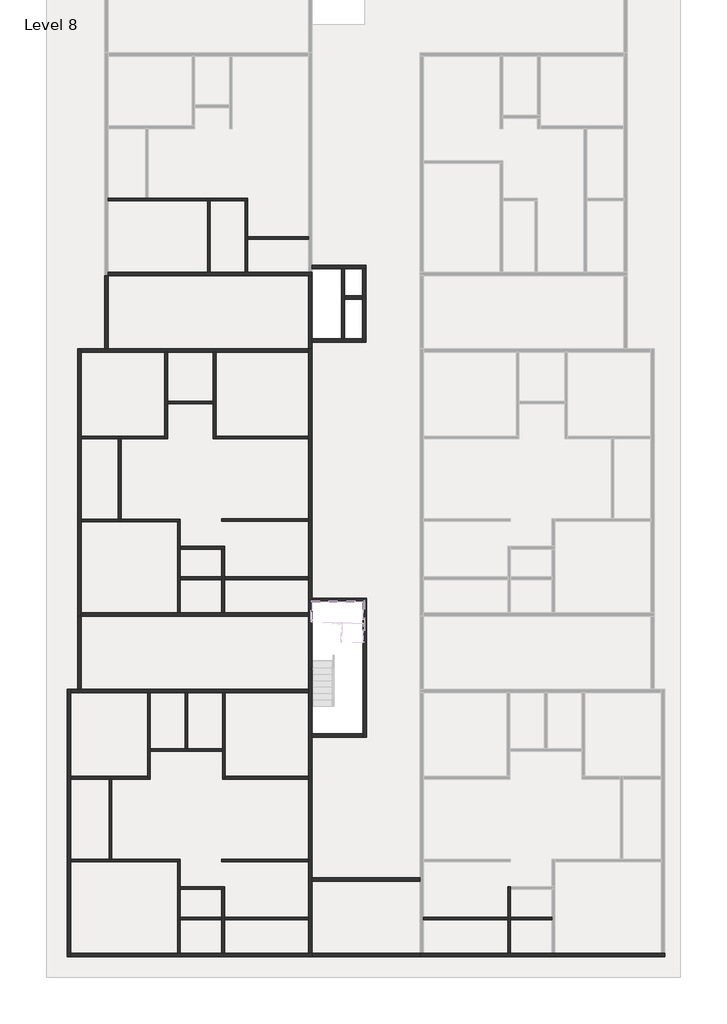
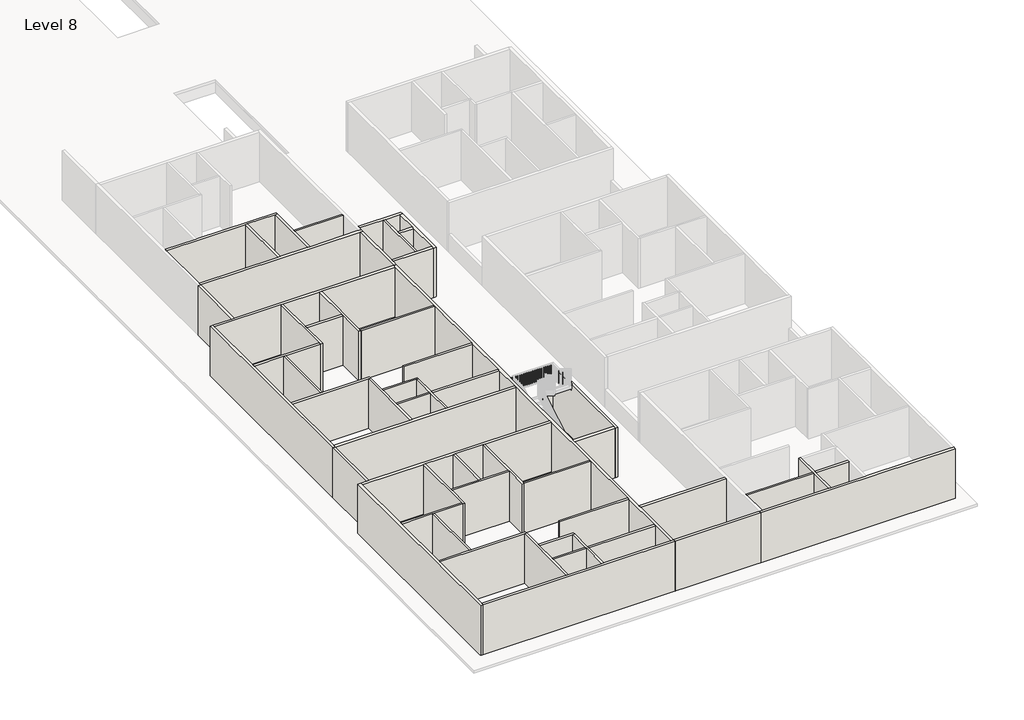
# One storey, part 1 of 8: 55 walls.
"""IFC4 building model written with IfcOpenShell, lengths in millimetres."""

from ifc_helpers import new_model, si_unit, frame, origin, place, context, project, spatial, polyline, outline, extrude, faceted_brep, element, save

model = new_model("IFC4")

# Units and contexts
model_context = context("Model", 3, world=origin())
ifc_project = project(units=[si_unit("LENGTHUNIT", "METRE", prefix="MILLI")], contexts=[model_context])

# Site, building, storey
site = spatial("IfcSite", under=ifc_project)
building = spatial("IfcBuilding", under=site)
storey = spatial("IfcBuildingStorey", under=building, Name="Level 8", Elevation=46570.6172466)

# Walls
placement = place(None, origin())
element("IfcWall", 1, ObjectType="4.5\"", at=placement, inside=storey, context=model_context, shape_type="Brep", body=[
    faceted_brep([(-12531.5544854, -1061.7344126, 46570.6172466), (-8188.1544854, -1061.7344126, 46570.6172466), (-8073.8544854, -1061.7344126, 46570.6172466), (-6549.8544854, -1061.7344126, 46570.6172466), (-6435.5544854, -1061.7344126, 46570.6172466), (-6435.5544854, -1061.7344126, 49618.6172466), (-6549.8544854, -1061.7344126, 49618.6172466), (-8073.8544854, -1061.7344126, 49618.6172466), (-8188.1544854, -1061.7344126, 49618.6172466), (-12531.5544854, -1061.7344126, 49618.6172466), (-12531.5544854, -947.4344126, 46570.6172466), (-12531.5544854, -947.4344126, 49618.6172466), (-10907.2415084, -947.4344126, 49618.6172466), (-10792.9415084, -947.4344126, 49618.6172466), (-6435.5544854, -947.4344126, 49618.6172466), (-6435.5544854, -947.4344126, 46570.6172466), (-10792.9415084, -947.4344126, 46570.6172466), (-10907.2415084, -947.4344126, 46570.6172466)], [[[0, 1, 2, 3, 4, 5, 6, 7, 8, 9]], [[10, 11, 12, 13, 14, 15, 16, 17]], [[4, 3, 2, 1, 0, 10, 17, 16, 15]], [[0, 9, 11, 10]], [[5, 4, 15, 14]], [[9, 8, 7, 6, 5, 14, 13, 12, 11]]]),
])
element("IfcWall", 2, ObjectType="4.5\"", at=placement, inside=storey, context=model_context, shape_type="Brep", body=[
    faceted_brep([(-6549.8544854, -1061.7344126, 46570.6172466), (-6549.8544854, -4185.9344126, 46570.6172466), (-6549.8544854, -4185.9344126, 49618.6172466), (-6549.8544854, -1061.7344126, 49618.6172466), (-6435.5544854, -1061.7344126, 46570.6172466), (-6435.5544854, -1061.7344126, 49618.6172466), (-6435.5544854, -2623.8344126, 49618.6172466), (-6435.5544854, -2738.1344126, 49618.6172466), (-6435.5544854, -4185.9344126, 49618.6172466), (-6435.5544854, -4185.9344126, 46570.6172466), (-6435.5544854, -2738.1344126, 46570.6172466), (-6435.5544854, -2623.8344126, 46570.6172466)], [[[0, 1, 2, 3]], [[4, 5, 6, 7, 8, 9, 10, 11]], [[1, 0, 4, 11, 10, 9]], [[0, 3, 5, 4]], [[2, 1, 9, 8]], [[3, 2, 8, 7, 6, 5]]]),
])
element("IfcWall", 3, ObjectType="4.5\"", at=placement, inside=storey, context=model_context, shape_type="SweptSolid", body=[
    extrude(outline(polyline([(-8188.1544854, -4185.9344126), (-8188.1544854, -1061.7344126), (-8073.8544854, -1061.7344126), (-8073.8544854, -4185.9344126), (-8188.1544854, -4185.9344126)])), frame((0.0, 0.0, 46570.6172466), z_axis=(0.0, 0.0, 1.0), x_axis=(1.0, 0.0, 0.0)), (0.0, 0.0, 1.0), 3048.0),
])
element("IfcWall", 4, ObjectType="4.5\"", at=placement, inside=storey, context=model_context, shape_type="SweptSolid", body=[
    extrude(outline(polyline([(-6435.5544854, -2623.8344126), (-3769.8415084, -2623.8344126), (-3769.8415084, -2738.1344126), (-6435.5544854, -2738.1344126), (-6435.5544854, -2623.8344126)])), frame((0.0, 0.0, 46570.6172466), z_axis=(0.0, 0.0, 1.0), x_axis=(1.0, 0.0, 0.0)), (0.0, 0.0, 1.0), 3048.0),
])
element("IfcWall", 5, ObjectType="4.5\"", at=placement, inside=storey, context=model_context, shape_type="Brep", body=[
    faceted_brep([(-10061.4044854, -7691.1344126, 46570.6172466), (-10061.4044854, -11348.7344126, 46570.6172466), (-10061.4044854, -11463.0344126, 46570.6172466), (-10061.4044854, -11463.0344126, 49618.6172466), (-10061.4044854, -11348.7344126, 49618.6172466), (-10061.4044854, -7691.1344126, 49618.6172466), (-9947.1044854, -7691.1344126, 46570.6172466), (-9947.1044854, -7691.1344126, 49618.6172466), (-9947.1044854, -9824.7344126, 49618.6172466), (-9947.1044854, -9939.0344126, 49618.6172466), (-9947.1044854, -11463.0344126, 49618.6172466), (-9947.1044854, -11463.0344126, 46570.6172466), (-9947.1044854, -9939.0344126, 46570.6172466), (-9947.1044854, -9824.7344126, 46570.6172466)], [[[0, 1, 2, 3, 4, 5]], [[6, 7, 8, 9, 10, 11, 12, 13]], [[2, 1, 0, 6, 13, 12, 11]], [[0, 5, 7, 6]], [[3, 2, 11, 10]], [[5, 4, 3, 10, 9, 8, 7]]]),
])
element("IfcWall", 6, ObjectType="4.5\"", at=placement, inside=storey, context=model_context, shape_type="Brep", body=[
    faceted_brep([(-10061.4044854, -11348.7344126, 46570.6172466), (-13719.0044854, -11348.7344126, 46570.6172466), (-13719.0044854, -11348.7344126, 49618.6172466), (-10061.4044854, -11348.7344126, 49618.6172466), (-10061.4044854, -11463.0344126, 46570.6172466), (-10061.4044854, -11463.0344126, 49618.6172466), (-11980.3915084, -11463.0344126, 49618.6172466), (-12094.6915084, -11463.0344126, 49618.6172466), (-13719.0044854, -11463.0344126, 49618.6172466), (-13719.0044854, -11463.0344126, 46570.6172466), (-12094.6915084, -11463.0344126, 46570.6172466), (-11980.3915084, -11463.0344126, 46570.6172466)], [[[0, 1, 2, 3]], [[4, 5, 6, 7, 8, 9, 10, 11]], [[1, 0, 4, 11, 10, 9]], [[0, 3, 5, 4]], [[2, 1, 9, 8]], [[3, 2, 8, 7, 6, 5]]]),
])
element("IfcWall", 7, ObjectType="4.5\"", at=placement, inside=storey, context=model_context, shape_type="SweptSolid", body=[
    extrude(outline(polyline([(-12094.6915084, -14968.2344126), (-12094.6915084, -11463.0344126), (-11980.3915084, -11463.0344126), (-11980.3915084, -14968.2344126), (-12094.6915084, -14968.2344126)])), frame((0.0, 0.0, 46570.6172466), z_axis=(0.0, 0.0, 1.0), x_axis=(1.0, 0.0, 0.0)), (0.0, 0.0, 1.0), 3048.0),
])
element("IfcWall", 8, ObjectType="4.5\"", at=placement, inside=storey, context=model_context, shape_type="Brep", body=[
    faceted_brep([(-13719.0044854, -15095.2344126, 46570.6172466), (-9510.2415084, -15095.2344126, 46570.6172466), (-9395.9415084, -15095.2344126, 46570.6172466), (-9395.9415084, -15095.2344126, 49618.6172466), (-9510.2415084, -15095.2344126, 49618.6172466), (-13719.0044854, -15095.2344126, 49618.6172466), (-13719.0044854, -14980.9344126, 46570.6172466), (-13719.0044854, -14980.9344126, 49618.6172466), (-9395.9415084, -14980.9344126, 49618.6172466), (-9395.9415084, -14980.9344126, 46570.6172466)], [[[0, 1, 2, 3, 4, 5]], [[6, 7, 8, 9]], [[2, 1, 0, 6, 9]], [[0, 5, 7, 6]], [[3, 2, 9, 8]], [[5, 4, 3, 8, 7]]]),
])
element("IfcWall", 9, ObjectType="4.5\"", at=placement, inside=storey, context=model_context, shape_type="Brep", body=[
    faceted_brep([(-9510.2415084, -15095.2344126, 46570.6172466), (-9510.2415084, -19070.3344126, 46570.6172466), (-9510.2415084, -19070.3344126, 49618.6172466), (-9510.2415084, -15095.2344126, 49618.6172466), (-9395.9415084, -15095.2344126, 46570.6172466), (-9395.9415084, -15095.2344126, 49618.6172466), (-9395.9415084, -16174.7344126, 49618.6172466), (-9395.9415084, -16289.0344126, 49618.6172466), (-9395.9415084, -17508.2344126, 49618.6172466), (-9395.9415084, -17622.5344126, 49618.6172466), (-9395.9415084, -19070.3344126, 49618.6172466), (-9395.9415084, -19070.3344126, 46570.6172466), (-9395.9415084, -17622.5344126, 46570.6172466), (-9395.9415084, -17508.2344126, 46570.6172466), (-9395.9415084, -16289.0344126, 46570.6172466), (-9395.9415084, -16174.7344126, 46570.6172466)], [[[0, 1, 2, 3]], [[4, 5, 6, 7, 8, 9, 10, 11, 12, 13, 14, 15]], [[1, 0, 4, 15, 14, 13, 12, 11]], [[0, 3, 5, 4]], [[2, 1, 11, 10]], [[3, 2, 10, 9, 8, 7, 6, 5]]]),
])
element("IfcWall", 10, ObjectType="4.5\"", at=placement, inside=storey, context=model_context, shape_type="Brep", body=[
    faceted_brep([(-9395.9415084, -16289.0344126, 46570.6172466), (-7567.1415084, -16289.0344126, 46570.6172466), (-7452.8415084, -16289.0344126, 46570.6172466), (-7452.8415084, -16289.0344126, 49618.6172466), (-7567.1415084, -16289.0344126, 49618.6172466), (-9395.9415084, -16289.0344126, 49618.6172466), (-9395.9415084, -16174.7344126, 46570.6172466), (-9395.9415084, -16174.7344126, 49618.6172466), (-7452.8415084, -16174.7344126, 49618.6172466), (-7452.8415084, -16174.7344126, 46570.6172466)], [[[0, 1, 2, 3, 4, 5]], [[6, 7, 8, 9]], [[2, 1, 0, 6, 9]], [[0, 5, 7, 6]], [[3, 2, 9, 8]], [[5, 4, 3, 8, 7]]]),
])
element("IfcWall", 11, ObjectType="4.5\"", at=placement, inside=storey, context=model_context, shape_type="Brep", body=[
    faceted_brep([(-7567.1415084, -16289.0344126, 46570.6172466), (-7567.1415084, -17508.2344126, 46570.6172466), (-7567.1415084, -17622.5344126, 46570.6172466), (-7567.1415084, -19070.3344126, 46570.6172466), (-7567.1415084, -19070.3344126, 49618.6172466), (-7567.1415084, -17622.5344126, 49618.6172466), (-7567.1415084, -17508.2344126, 49618.6172466), (-7567.1415084, -16289.0344126, 49618.6172466), (-7452.8415084, -16289.0344126, 46570.6172466), (-7452.8415084, -16289.0344126, 49618.6172466), (-7452.8415084, -17508.2344126, 49618.6172466), (-7452.8415084, -17622.5344126, 49618.6172466), (-7452.8415084, -19070.3344126, 49618.6172466), (-7452.8415084, -19070.3344126, 46570.6172466), (-7452.8415084, -17622.5344126, 46570.6172466), (-7452.8415084, -17508.2344126, 46570.6172466)], [[[0, 1, 2, 3, 4, 5, 6, 7]], [[8, 9, 10, 11, 12, 13, 14, 15]], [[3, 2, 1, 0, 8, 15, 14, 13]], [[0, 7, 9, 8]], [[4, 3, 13, 12]], [[7, 6, 5, 4, 12, 11, 10, 9]]]),
])
element("IfcWall", 12, ObjectType="4.5\"", at=placement, inside=storey, context=model_context, shape_type="SweptSolid", body=[
    extrude(outline(polyline([(-7567.1415084, -17622.5344126), (-9395.9415084, -17622.5344126), (-9395.9415084, -17508.2344126), (-7567.1415084, -17508.2344126), (-7567.1415084, -17622.5344126)])), frame((0.0, 0.0, 46570.6172466), z_axis=(0.0, 0.0, 1.0), x_axis=(1.0, 0.0, 0.0)), (0.0, 0.0, 1.0), 3048.0),
])
element("IfcWall", 13, ObjectType="4.5\"", at=placement, inside=storey, context=model_context, shape_type="SweptSolid", body=[
    extrude(outline(polyline([(-3769.8415084, -17622.5344126), (-7452.8415084, -17622.5344126), (-7452.8415084, -17508.2344126), (-3769.8415084, -17508.2344126), (-3769.8415084, -17622.5344126)])), frame((0.0, 0.0, 46570.6172466), z_axis=(0.0, 0.0, 1.0), x_axis=(1.0, 0.0, 0.0)), (0.0, 0.0, 1.0), 3048.0),
])
element("IfcWall", 14, ObjectType="4.5\"", at=placement, inside=storey, context=model_context, shape_type="SweptSolid", body=[
    extrude(outline(polyline([(-7567.1415084, -14968.2344126), (-3769.8415084, -14968.2344126), (-3769.8415084, -15082.5344126), (-7567.1415084, -15082.5344126), (-7567.1415084, -14968.2344126)])), frame((0.0, 0.0, 46570.6172466), z_axis=(0.0, 0.0, 1.0), x_axis=(1.0, 0.0, 0.0)), (0.0, 0.0, 1.0), 3048.0),
])
element("IfcWall", 15, ObjectType="4.5\"", at=placement, inside=storey, context=model_context, shape_type="SweptSolid", body=[
    extrude(outline(polyline([(-7940.5044854, -9939.0344126), (-9947.1044854, -9939.0344126), (-9947.1044854, -9824.7344126), (-7940.5044854, -9824.7344126), (-7940.5044854, -9939.0344126)])), frame((0.0, 0.0, 46570.6172466), z_axis=(0.0, 0.0, 1.0), x_axis=(1.0, 0.0, 0.0)), (0.0, 0.0, 1.0), 3048.0),
])
element("IfcWall", 16, ObjectType="4.5\"", at=placement, inside=storey, context=model_context, shape_type="Brep", body=[
    faceted_brep([(-7940.5044854, -7691.1344126, 46570.6172466), (-7940.5044854, -9824.7344126, 46570.6172466), (-7940.5044854, -9939.0344126, 46570.6172466), (-7940.5044854, -11463.0344126, 46570.6172466), (-7940.5044854, -11463.0344126, 49618.6172466), (-7940.5044854, -9939.0344126, 49618.6172466), (-7940.5044854, -9824.7344126, 49618.6172466), (-7940.5044854, -7691.1344126, 49618.6172466), (-7826.2044854, -7691.1344126, 46570.6172466), (-7826.2044854, -7691.1344126, 49618.6172466), (-7826.2044854, -11348.7344126, 49618.6172466), (-7826.2044854, -11463.0344126, 49618.6172466), (-7826.2044854, -11463.0344126, 46570.6172466), (-7826.2044854, -11348.7344126, 46570.6172466)], [[[0, 1, 2, 3, 4, 5, 6, 7]], [[8, 9, 10, 11, 12, 13]], [[3, 2, 1, 0, 8, 13, 12]], [[0, 7, 9, 8]], [[4, 3, 12, 11]], [[7, 6, 5, 4, 11, 10, 9]]]),
])
element("IfcWall", 17, ObjectType="4.5\"", at=placement, inside=storey, context=model_context, shape_type="SweptSolid", body=[
    extrude(outline(polyline([(-3769.8415084, -11463.0344126), (-7826.2044854, -11463.0344126), (-7826.2044854, -11348.7344126), (-3769.8415084, -11348.7344126), (-3769.8415084, -11463.0344126)])), frame((0.0, 0.0, 46570.6172466), z_axis=(0.0, 0.0, 1.0), x_axis=(1.0, 0.0, 0.0)), (0.0, 0.0, 1.0), 3048.0),
])
element("IfcWall", 18, ObjectType="4.5\"", at=placement, inside=storey, context=model_context, shape_type="Brep", body=[
    faceted_brep([(-10818.3415084, -22575.5344126, 46570.6172466), (-10818.3415084, -26233.1344126, 46570.6172466), (-10818.3415084, -26347.4344126, 46570.6172466), (-10818.3415084, -26347.4344126, 49618.6172466), (-10818.3415084, -26233.1344126, 49618.6172466), (-10818.3415084, -22575.5344126, 49618.6172466), (-10704.0415084, -22575.5344126, 46570.6172466), (-10704.0415084, -22575.5344126, 49618.6172466), (-10704.0415084, -25013.9344126, 49618.6172466), (-10704.0415084, -25128.2344126, 49618.6172466), (-10704.0415084, -26347.4344126, 49618.6172466), (-10704.0415084, -26347.4344126, 46570.6172466), (-10704.0415084, -25128.2344126, 46570.6172466), (-10704.0415084, -25013.9344126, 46570.6172466)], [[[0, 1, 2, 3, 4, 5]], [[6, 7, 8, 9, 10, 11, 12, 13]], [[2, 1, 0, 6, 13, 12, 11]], [[0, 5, 7, 6]], [[3, 2, 11, 10]], [[5, 4, 3, 10, 9, 8, 7]]]),
])
element("IfcWall", 19, ObjectType="4.5\"", at=placement, inside=storey, context=model_context, shape_type="Brep", body=[
    faceted_brep([(-10818.3415084, -26233.1344126, 46570.6172466), (-14171.1415084, -26233.1344126, 46570.6172466), (-14171.1415084, -26233.1344126, 49618.6172466), (-10818.3415084, -26233.1344126, 49618.6172466), (-10818.3415084, -26347.4344126, 46570.6172466), (-10818.3415084, -26347.4344126, 49618.6172466), (-12380.4415084, -26347.4344126, 49618.6172466), (-12494.7415084, -26347.4344126, 49618.6172466), (-14171.1415084, -26347.4344126, 49618.6172466), (-14171.1415084, -26347.4344126, 46570.6172466), (-12494.7415084, -26347.4344126, 46570.6172466), (-12380.4415084, -26347.4344126, 46570.6172466)], [[[0, 1, 2, 3]], [[4, 5, 6, 7, 8, 9, 10, 11]], [[1, 0, 4, 11, 10, 9]], [[0, 3, 5, 4]], [[2, 1, 9, 8]], [[3, 2, 8, 7, 6, 5]]]),
])
element("IfcWall", 20, ObjectType="4.5\"", at=placement, inside=storey, context=model_context, shape_type="SweptSolid", body=[
    extrude(outline(polyline([(-9180.0415084, -25013.9344126), (-9180.0415084, -22575.5344126), (-9065.7415084, -22575.5344126), (-9065.7415084, -25013.9344126), (-9180.0415084, -25013.9344126)])), frame((0.0, 0.0, 46570.6172466), z_axis=(0.0, 0.0, 1.0), x_axis=(1.0, 0.0, 0.0)), (0.0, 0.0, 1.0), 3048.0),
])
element("IfcWall", 21, ObjectType="4.5\"", at=placement, inside=storey, context=model_context, shape_type="Brep", body=[
    faceted_brep([(-10704.0415084, -25128.2344126, 46570.6172466), (-7541.7415084, -25128.2344126, 46570.6172466), (-7541.7415084, -25128.2344126, 49618.6172466), (-10704.0415084, -25128.2344126, 49618.6172466), (-10704.0415084, -25013.9344126, 46570.6172466), (-10704.0415084, -25013.9344126, 49618.6172466), (-9180.0415084, -25013.9344126, 49618.6172466), (-9065.7415084, -25013.9344126, 49618.6172466), (-7541.7415084, -25013.9344126, 49618.6172466), (-7541.7415084, -25013.9344126, 46570.6172466), (-9065.7415084, -25013.9344126, 46570.6172466), (-9180.0415084, -25013.9344126, 46570.6172466)], [[[0, 1, 2, 3]], [[4, 5, 6, 7, 8, 9, 10, 11]], [[1, 0, 4, 11, 10, 9]], [[0, 3, 5, 4]], [[2, 1, 9, 8]], [[3, 2, 8, 7, 6, 5]]]),
])
element("IfcWall", 22, ObjectType="4.5\"", at=placement, inside=storey, context=model_context, shape_type="Brep", body=[
    faceted_brep([(-7541.7415084, -22575.5344126, 46570.6172466), (-7541.7415084, -25013.9344126, 46570.6172466), (-7541.7415084, -25128.2344126, 46570.6172466), (-7541.7415084, -26347.4344126, 46570.6172466), (-7541.7415084, -26347.4344126, 49618.6172466), (-7541.7415084, -25128.2344126, 49618.6172466), (-7541.7415084, -25013.9344126, 49618.6172466), (-7541.7415084, -22575.5344126, 49618.6172466), (-7427.4415084, -22575.5344126, 46570.6172466), (-7427.4415084, -22575.5344126, 49618.6172466), (-7427.4415084, -26233.1344126, 49618.6172466), (-7427.4415084, -26347.4344126, 49618.6172466), (-7427.4415084, -26347.4344126, 46570.6172466), (-7427.4415084, -26233.1344126, 46570.6172466)], [[[0, 1, 2, 3, 4, 5, 6, 7]], [[8, 9, 10, 11, 12, 13]], [[3, 2, 1, 0, 8, 13, 12]], [[0, 7, 9, 8]], [[4, 3, 12, 11]], [[7, 6, 5, 4, 11, 10, 9]]]),
])
element("IfcWall", 23, ObjectType="4.5\"", at=placement, inside=storey, context=model_context, shape_type="SweptSolid", body=[
    extrude(outline(polyline([(-3769.8415084, -26347.4344126), (-7427.4415084, -26347.4344126), (-7427.4415084, -26233.1344126), (-3769.8415084, -26233.1344126), (-3769.8415084, -26347.4344126)])), frame((0.0, 0.0, 46570.6172466), z_axis=(0.0, 0.0, 1.0), x_axis=(1.0, 0.0, 0.0)), (0.0, 0.0, 1.0), 3048.0),
])
element("IfcWall", 24, ObjectType="4.5\"", at=placement, inside=storey, context=model_context, shape_type="SweptSolid", body=[
    extrude(outline(polyline([(-12494.7415084, -29852.6344126), (-12494.7415084, -26347.4344126), (-12380.4415084, -26347.4344126), (-12380.4415084, -29852.6344126), (-12494.7415084, -29852.6344126)])), frame((0.0, 0.0, 46570.6172466), z_axis=(0.0, 0.0, 1.0), x_axis=(1.0, 0.0, 0.0)), (0.0, 0.0, 1.0), 3048.0),
])
element("IfcWall", 25, ObjectType="4.5\"", at=placement, inside=storey, context=model_context, shape_type="Brep", body=[
    faceted_brep([(-14171.1415084, -29966.9344126, 46570.6172466), (-9510.2415084, -29966.9344126, 46570.6172466), (-9395.9415084, -29966.9344126, 46570.6172466), (-9395.9415084, -29966.9344126, 49618.6172466), (-9510.2415084, -29966.9344126, 49618.6172466), (-14171.1415084, -29966.9344126, 49618.6172466), (-14171.1415084, -29852.6344126, 46570.6172466), (-14171.1415084, -29852.6344126, 49618.6172466), (-12494.7415084, -29852.6344126, 49618.6172466), (-12380.4415084, -29852.6344126, 49618.6172466), (-9395.9415084, -29852.6344126, 49618.6172466), (-9395.9415084, -29852.6344126, 46570.6172466), (-12380.4415084, -29852.6344126, 46570.6172466), (-12494.7415084, -29852.6344126, 46570.6172466)], [[[0, 1, 2, 3, 4, 5]], [[6, 7, 8, 9, 10, 11, 12, 13]], [[2, 1, 0, 6, 13, 12, 11]], [[0, 5, 7, 6]], [[3, 2, 11, 10]], [[5, 4, 3, 10, 9, 8, 7]]]),
])
element("IfcWall", 26, ObjectType="4.5\"", at=placement, inside=storey, context=model_context, shape_type="Brep", body=[
    faceted_brep([(-9510.2415084, -29966.9344126, 46570.6172466), (-9510.2415084, -33954.7344126, 46570.6172466), (-9510.2415084, -33954.7344126, 49618.6172466), (-9510.2415084, -29966.9344126, 49618.6172466), (-9395.9415084, -29966.9344126, 46570.6172466), (-9395.9415084, -29966.9344126, 49618.6172466), (-9395.9415084, -31059.1344126, 49618.6172466), (-9395.9415084, -31173.4344126, 49618.6172466), (-9395.9415084, -32392.6344126, 49618.6172466), (-9395.9415084, -32506.9344126, 49618.6172466), (-9395.9415084, -33954.7344126, 49618.6172466), (-9395.9415084, -33954.7344126, 46570.6172466), (-9395.9415084, -32506.9344126, 46570.6172466), (-9395.9415084, -32392.6344126, 46570.6172466), (-9395.9415084, -31173.4344126, 46570.6172466), (-9395.9415084, -31059.1344126, 46570.6172466)], [[[0, 1, 2, 3]], [[4, 5, 6, 7, 8, 9, 10, 11, 12, 13, 14, 15]], [[1, 0, 4, 15, 14, 13, 12, 11]], [[0, 3, 5, 4]], [[2, 1, 11, 10]], [[3, 2, 10, 9, 8, 7, 6, 5]]]),
])
element("IfcWall", 27, ObjectType="4.5\"", at=placement, inside=storey, context=model_context, shape_type="Brep", body=[
    faceted_brep([(-9395.9415084, -31173.4344126, 46570.6172466), (-7567.1415084, -31173.4344126, 46570.6172466), (-7452.8415084, -31173.4344126, 46570.6172466), (-7452.8415084, -31173.4344126, 49618.6172466), (-7567.1415084, -31173.4344126, 49618.6172466), (-9395.9415084, -31173.4344126, 49618.6172466), (-9395.9415084, -31059.1344126, 46570.6172466), (-9395.9415084, -31059.1344126, 49618.6172466), (-7452.8415084, -31059.1344126, 49618.6172466), (-7452.8415084, -31059.1344126, 46570.6172466)], [[[0, 1, 2, 3, 4, 5]], [[6, 7, 8, 9]], [[2, 1, 0, 6, 9]], [[0, 5, 7, 6]], [[3, 2, 9, 8]], [[5, 4, 3, 8, 7]]]),
])
element("IfcWall", 28, ObjectType="4.5\"", at=placement, inside=storey, context=model_context, shape_type="Brep", body=[
    faceted_brep([(-7567.1415084, -31173.4344126, 46570.6172466), (-7567.1415084, -32392.6344126, 46570.6172466), (-7567.1415084, -32506.9344126, 46570.6172466), (-7567.1415084, -33954.7344126, 46570.6172466), (-7567.1415084, -33954.7344126, 49618.6172466), (-7567.1415084, -32506.9344126, 49618.6172466), (-7567.1415084, -32392.6344126, 49618.6172466), (-7567.1415084, -31173.4344126, 49618.6172466), (-7452.8415084, -31173.4344126, 46570.6172466), (-7452.8415084, -31173.4344126, 49618.6172466), (-7452.8415084, -32392.6344126, 49618.6172466), (-7452.8415084, -32506.9344126, 49618.6172466), (-7452.8415084, -33954.7344126, 49618.6172466), (-7452.8415084, -33954.7344126, 46570.6172466), (-7452.8415084, -32506.9344126, 46570.6172466), (-7452.8415084, -32392.6344126, 46570.6172466)], [[[0, 1, 2, 3, 4, 5, 6, 7]], [[8, 9, 10, 11, 12, 13, 14, 15]], [[3, 2, 1, 0, 8, 15, 14, 13]], [[0, 7, 9, 8]], [[4, 3, 13, 12]], [[7, 6, 5, 4, 12, 11, 10, 9]]]),
])
element("IfcWall", 29, ObjectType="4.5\"", at=placement, inside=storey, context=model_context, shape_type="SweptSolid", body=[
    extrude(outline(polyline([(-3769.8415084, -32392.6344126), (-3769.8415084, -32506.9344126), (-7452.8415084, -32506.9344126), (-7452.8415084, -32392.6344126), (-3769.8415084, -32392.6344126)])), frame((0.0, 0.0, 46570.6172466), z_axis=(0.0, 0.0, 1.0), x_axis=(1.0, 0.0, 0.0)), (0.0, 0.0, 1.0), 3048.0),
    extrude(outline(polyline([(-9395.9415084, -32506.9344126), (-9395.9415084, -32392.6344126), (-7567.1415084, -32392.6344126), (-7567.1415084, -32506.9344126), (-9395.9415084, -32506.9344126)])), frame((0.0, 0.0, 46570.6172466), z_axis=(0.0, 0.0, 1.0), x_axis=(1.0, 0.0, 0.0)), (0.0, 0.0, 1.0), 3048.0),
])
element("IfcWall", 30, ObjectType="4.5\"", at=placement, inside=storey, context=model_context, shape_type="SweptSolid", body=[
    extrude(outline(polyline([(-7567.1415084, -29852.6344126), (-3769.8415084, -29852.6344126), (-3769.8415084, -29966.9344126), (-7567.1415084, -29966.9344126), (-7567.1415084, -29852.6344126)])), frame((0.0, 0.0, 46570.6172466), z_axis=(0.0, 0.0, 1.0), x_axis=(1.0, 0.0, 0.0)), (0.0, 0.0, 1.0), 3048.0),
])
element("IfcWall", 31, ObjectType="4.5\"", at=placement, inside=storey, context=model_context, shape_type="SweptSolid", body=[
    extrude(outline(polyline([(4942.3584916, -32506.9344126), (1259.3584916, -32506.9344126), (1259.3584916, -32392.6344126), (4942.3584916, -32392.6344126), (4942.3584916, -32506.9344126)])), frame((0.0, 0.0, 46570.6172466), z_axis=(0.0, 0.0, 1.0), x_axis=(1.0, 0.0, 0.0)), (0.0, 0.0, 1.0), 3048.0),
])
element("IfcWall", 32, ObjectType="4.5\"", at=placement, inside=storey, context=model_context, shape_type="Brep", body=[
    faceted_brep([(4942.3584916, -31059.1344126, 46570.6172466), (4942.3584916, -32392.6344126, 46570.6172466), (4942.3584916, -32506.9344126, 46570.6172466), (4942.3584916, -33954.7344126, 46570.6172466), (4942.3584916, -33954.7344126, 49618.6172466), (4942.3584916, -32506.9344126, 49618.6172466), (4942.3584916, -32392.6344126, 49618.6172466), (4942.3584916, -31059.1344126, 49618.6172466), (5056.6584916, -31059.1344126, 46570.6172466), (5056.6584916, -31059.1344126, 49618.6172466), (5056.6584916, -31173.4344126, 49618.6172466), (5056.6584916, -32392.6344126, 49618.6172466), (5056.6584916, -32506.9344126, 49618.6172466), (5056.6584916, -33954.7344126, 49618.6172466), (5056.6584916, -33954.7344126, 46570.6172466), (5056.6584916, -32506.9344126, 46570.6172466), (5056.6584916, -32392.6344126, 46570.6172466), (5056.6584916, -31173.4344126, 46570.6172466)], [[[0, 1, 2, 3, 4, 5, 6, 7]], [[8, 9, 10, 11, 12, 13, 14, 15, 16, 17]], [[3, 2, 1, 0, 8, 17, 16, 15, 14]], [[4, 3, 14, 13]], [[0, 7, 9, 8]], [[7, 6, 5, 4, 13, 12, 11, 10, 9]]]),
])
element("IfcWall", 33, ObjectType="4.5\"", at=placement, inside=storey, context=model_context, shape_type="SweptSolid", body=[
    extrude(outline(polyline([(6885.4584916, -32506.9344126), (5056.6584916, -32506.9344126), (5056.6584916, -32392.6344126), (6885.4584916, -32392.6344126), (6885.4584916, -32506.9344126)])), frame((0.0, 0.0, 46570.6172466), z_axis=(0.0, 0.0, 1.0), x_axis=(1.0, 0.0, 0.0)), (0.0, 0.0, 1.0), 3048.0),
])
element("IfcWall", 34, ObjectType="4.5\"", at=placement, inside=storey, context=model_context, shape_type="Brep", body=[
    faceted_brep([(-2207.6738684, -7082.6751812, 46570.6172466), (-2207.6738684, -5366.3479894, 46570.6172466), (-2207.6738684, -5213.9479894, 46570.6172466), (-2207.6738684, -4034.6751812, 46570.6172466), (-2207.6738684, -4034.6751812, 49618.6172466), (-2207.6738684, -5213.9479894, 49618.6172466), (-2207.6738684, -5366.3479894, 49618.6172466), (-2207.6738684, -7082.6751812, 49618.6172466), (-2321.9738684, -7082.6751812, 46570.6172466), (-2321.9738684, -7082.6751812, 49618.6172466), (-2321.9738684, -4034.6751812, 49618.6172466), (-2321.9738684, -4034.6751812, 46570.6172466)], [[[0, 1, 2, 3, 4, 5, 6, 7]], [[8, 9, 10, 11]], [[3, 2, 1, 0, 8, 11]], [[7, 6, 5, 4, 10, 9]], [[4, 3, 11, 10]], [[0, 7, 9, 8]]]),
])
element("IfcWall", 35, ObjectType="6\"", at=placement, inside=storey, context=model_context, shape_type="Brep", body=[
    faceted_brep([(-12531.5544854, -4338.3344126, 46570.6172466), (-3769.8415084, -4338.3344126, 46570.6172466), (-3617.4415084, -4338.3344126, 46570.6172466), (-3617.4415084, -4338.3344126, 49618.6172466), (-3769.8415084, -4338.3344126, 49618.6172466), (-12531.5544854, -4338.3344126, 49618.6172466), (-12531.5544854, -4185.9344126, 46570.6172466), (-12531.5544854, -4185.9344126, 49618.6172466), (-8188.1544854, -4185.9344126, 49618.6172466), (-8073.8544854, -4185.9344126, 49618.6172466), (-6549.8544854, -4185.9344126, 49618.6172466), (-6435.5544854, -4185.9344126, 49618.6172466), (-3769.8415084, -4185.9344126, 49618.6172466), (-3617.4415084, -4185.9344126, 49618.6172466), (-3617.4415084, -4185.9344126, 46570.6172466), (-3769.8415084, -4185.9344126, 46570.6172466), (-6435.5544854, -4185.9344126, 46570.6172466), (-6549.8544854, -4185.9344126, 46570.6172466), (-8073.8544854, -4185.9344126, 46570.6172466), (-8188.1544854, -4185.9344126, 46570.6172466)], [[[0, 1, 2, 3, 4, 5]], [[6, 7, 8, 9, 10, 11, 12, 13, 14, 15, 16, 17, 18, 19]], [[2, 1, 0, 6, 19, 18, 17, 16, 15, 14]], [[0, 5, 7, 6]], [[3, 2, 14, 13]], [[5, 4, 3, 13, 12, 11, 10, 9, 8, 7]]]),
])
element("IfcWall", 36, ObjectType="6\"", at=placement, inside=storey, context=model_context, shape_type="Brep", body=[
    faceted_brep([(-13871.4044854, -7538.7344126, 46570.6172466), (-13871.4044854, -19222.7344126, 46570.6172466), (-13871.4044854, -19222.7344126, 49618.6172466), (-13871.4044854, -7538.7344126, 49618.6172466), (-13719.0044854, -7538.7344126, 46570.6172466), (-13719.0044854, -7538.7344126, 49618.6172466), (-13719.0044854, -7691.1344126, 49618.6172466), (-13719.0044854, -11348.7344126, 49618.6172466), (-13719.0044854, -11463.0344126, 49618.6172466), (-13719.0044854, -14980.9344126, 49618.6172466), (-13719.0044854, -15095.2344126, 49618.6172466), (-13719.0044854, -19070.3344126, 49618.6172466), (-13719.0044854, -19222.7344126, 49618.6172466), (-13719.0044854, -19222.7344126, 46570.6172466), (-13719.0044854, -19070.3344126, 46570.6172466), (-13719.0044854, -15095.2344126, 46570.6172466), (-13719.0044854, -14980.9344126, 46570.6172466), (-13719.0044854, -11463.0344126, 46570.6172466), (-13719.0044854, -11348.7344126, 46570.6172466), (-13719.0044854, -7691.1344126, 46570.6172466)], [[[0, 1, 2, 3]], [[4, 5, 6, 7, 8, 9, 10, 11, 12, 13, 14, 15, 16, 17, 18, 19]], [[1, 0, 4, 19, 18, 17, 16, 15, 14, 13]], [[2, 1, 13, 12]], [[0, 3, 5, 4]], [[3, 2, 12, 11, 10, 9, 8, 7, 6, 5]]]),
])
element("IfcWall", 37, ObjectType="6\"", at=placement, inside=storey, context=model_context, shape_type="Brep", body=[
    faceted_brep([(-13719.0044854, -19222.7344126, 46570.6172466), (-3769.8415084, -19222.7344126, 46570.6172466), (-3769.8415084, -19222.7344126, 49618.6172466), (-13719.0044854, -19222.7344126, 49618.6172466), (-13719.0044854, -19070.3344126, 46570.6172466), (-13719.0044854, -19070.3344126, 49618.6172466), (-9510.2415084, -19070.3344126, 49618.6172466), (-9395.9415084, -19070.3344126, 49618.6172466), (-7567.1415084, -19070.3344126, 49618.6172466), (-7452.8415084, -19070.3344126, 49618.6172466), (-3769.8415084, -19070.3344126, 49618.6172466), (-3769.8415084, -19070.3344126, 46570.6172466), (-7452.8415084, -19070.3344126, 46570.6172466), (-7567.1415084, -19070.3344126, 46570.6172466), (-9395.9415084, -19070.3344126, 46570.6172466), (-9510.2415084, -19070.3344126, 46570.6172466)], [[[0, 1, 2, 3]], [[4, 5, 6, 7, 8, 9, 10, 11, 12, 13, 14, 15]], [[1, 0, 4, 15, 14, 13, 12, 11]], [[0, 3, 5, 4]], [[2, 1, 11, 10]], [[3, 2, 10, 9, 8, 7, 6, 5]]]),
])
element("IfcWall", 38, ObjectType="6\"", at=placement, inside=storey, context=model_context, shape_type="Brep", body=[
    faceted_brep([(-3617.4415084, -33954.7344126, 46570.6172466), (-3617.4415084, -30820.9325185, 46570.6172466), (-3617.4415084, -30668.5325185, 46570.6172466), (-3617.4415084, -24525.9851539, 46570.6172466), (-3617.4415084, -24373.5851539, 46570.6172466), (-3617.4415084, -18582.3851539, 46570.6172466), (-3617.4415084, -18429.9851539, 46570.6172466), (-3617.4415084, -7538.7344126, 46570.6172466), (-3617.4415084, -7538.7344126, 49618.6172466), (-3617.4415084, -18429.9851539, 49618.6172466), (-3617.4415084, -18582.3851539, 49618.6172466), (-3617.4415084, -24373.5851539, 49618.6172466), (-3617.4415084, -24525.9851539, 49618.6172466), (-3617.4415084, -30668.5325185, 49618.6172466), (-3617.4415084, -30820.9325185, 49618.6172466), (-3617.4415084, -33954.7344126, 49618.6172466), (-3769.8415084, -33954.7344126, 46570.6172466), (-3769.8415084, -33954.7344126, 49618.6172466), (-3769.8415084, -32506.9344126, 49618.6172466), (-3769.8415084, -32392.6344126, 49618.6172466), (-3769.8415084, -29966.9344126, 49618.6172466), (-3769.8415084, -29852.6344126, 49618.6172466), (-3769.8415084, -26347.4344126, 49618.6172466), (-3769.8415084, -26233.1344126, 49618.6172466), (-3769.8415084, -22575.5344126, 49618.6172466), (-3769.8415084, -22423.1344126, 49618.6172466), (-3769.8415084, -19222.7344126, 49618.6172466), (-3769.8415084, -19070.3344126, 49618.6172466), (-3769.8415084, -17622.5344126, 49618.6172466), (-3769.8415084, -17508.2344126, 49618.6172466), (-3769.8415084, -15082.5344126, 49618.6172466), (-3769.8415084, -14968.2344126, 49618.6172466), (-3769.8415084, -11463.0344126, 49618.6172466), (-3769.8415084, -11348.7344126, 49618.6172466), (-3769.8415084, -7691.1344126, 49618.6172466), (-3769.8415084, -7538.7344126, 49618.6172466), (-3769.8415084, -7538.7344126, 46570.6172466), (-3769.8415084, -7691.1344126, 46570.6172466), (-3769.8415084, -11348.7344126, 46570.6172466), (-3769.8415084, -11463.0344126, 46570.6172466), (-3769.8415084, -14968.2344126, 46570.6172466), (-3769.8415084, -15082.5344126, 46570.6172466), (-3769.8415084, -17508.2344126, 46570.6172466), (-3769.8415084, -17622.5344126, 46570.6172466), (-3769.8415084, -19070.3344126, 46570.6172466), (-3769.8415084, -19222.7344126, 46570.6172466), (-3769.8415084, -22423.1344126, 46570.6172466), (-3769.8415084, -22575.5344126, 46570.6172466), (-3769.8415084, -26233.1344126, 46570.6172466), (-3769.8415084, -26347.4344126, 46570.6172466), (-3769.8415084, -29852.6344126, 46570.6172466), (-3769.8415084, -29966.9344126, 46570.6172466), (-3769.8415084, -32392.6344126, 46570.6172466), (-3769.8415084, -32506.9344126, 46570.6172466)], [[[0, 1, 2, 3, 4, 5, 6, 7, 8, 9, 10, 11, 12, 13, 14, 15]], [[16, 17, 18, 19, 20, 21, 22, 23, 24, 25, 26, 27, 28, 29, 30, 31, 32, 33, 34, 35, 36, 37, 38, 39, 40, 41, 42, 43, 44, 45, 46, 47, 48, 49, 50, 51, 52, 53]], [[7, 6, 5, 4, 3, 2, 1, 0, 16, 53, 52, 51, 50, 49, 48, 47, 46, 45, 44, 43, 42, 41, 40, 39, 38, 37, 36]], [[8, 7, 36, 35]], [[0, 15, 17, 16]], [[15, 14, 13, 12, 11, 10, 9, 8, 35, 34, 33, 32, 31, 30, 29, 28, 27, 26, 25, 24, 23, 22, 21, 20, 19, 18, 17]]]),
])
element("IfcWall", 39, ObjectType="6\"", at=placement, inside=storey, context=model_context, shape_type="Brep", body=[
    faceted_brep([(-3769.8415084, -7538.7344126, 46570.6172466), (-12531.5544854, -7538.7344126, 46570.6172466), (-12683.9544854, -7538.7344126, 46570.6172466), (-13719.0044854, -7538.7344126, 46570.6172466), (-13719.0044854, -7538.7344126, 49618.6172466), (-12683.9544854, -7538.7344126, 49618.6172466), (-12531.5544854, -7538.7344126, 49618.6172466), (-3769.8415084, -7538.7344126, 49618.6172466), (-3769.8415084, -7691.1344126, 46570.6172466), (-3769.8415084, -7691.1344126, 49618.6172466), (-7826.2044854, -7691.1344126, 49618.6172466), (-7940.5044854, -7691.1344126, 49618.6172466), (-9947.1044854, -7691.1344126, 49618.6172466), (-10061.4044854, -7691.1344126, 49618.6172466), (-13719.0044854, -7691.1344126, 49618.6172466), (-13719.0044854, -7691.1344126, 46570.6172466), (-10061.4044854, -7691.1344126, 46570.6172466), (-9947.1044854, -7691.1344126, 46570.6172466), (-7940.5044854, -7691.1344126, 46570.6172466), (-7826.2044854, -7691.1344126, 46570.6172466)], [[[0, 1, 2, 3, 4, 5, 6, 7]], [[8, 9, 10, 11, 12, 13, 14, 15, 16, 17, 18, 19]], [[3, 2, 1, 0, 8, 19, 18, 17, 16, 15]], [[0, 7, 9, 8]], [[4, 3, 15, 14]], [[7, 6, 5, 4, 14, 13, 12, 11, 10, 9]]]),
])
element("IfcWall", 40, ObjectType="6\"", at=placement, inside=storey, context=model_context, shape_type="Brep", body=[
    faceted_brep([(-14323.5415084, -22423.1344126, 46570.6172466), (-14323.5415084, -34107.1344126, 46570.6172466), (-14323.5415084, -34107.1344126, 49618.6172466), (-14323.5415084, -22423.1344126, 49618.6172466), (-14171.1415084, -22423.1344126, 46570.6172466), (-14171.1415084, -22423.1344126, 49618.6172466), (-14171.1415084, -22575.5344126, 49618.6172466), (-14171.1415084, -26233.1344126, 49618.6172466), (-14171.1415084, -26347.4344126, 49618.6172466), (-14171.1415084, -29852.6344126, 49618.6172466), (-14171.1415084, -29966.9344126, 49618.6172466), (-14171.1415084, -33954.7344126, 49618.6172466), (-14171.1415084, -34107.1344126, 49618.6172466), (-14171.1415084, -34107.1344126, 46570.6172466), (-14171.1415084, -33954.7344126, 46570.6172466), (-14171.1415084, -29966.9344126, 46570.6172466), (-14171.1415084, -29852.6344126, 46570.6172466), (-14171.1415084, -26347.4344126, 46570.6172466), (-14171.1415084, -26233.1344126, 46570.6172466), (-14171.1415084, -22575.5344126, 46570.6172466)], [[[0, 1, 2, 3]], [[4, 5, 6, 7, 8, 9, 10, 11, 12, 13, 14, 15, 16, 17, 18, 19]], [[1, 0, 4, 19, 18, 17, 16, 15, 14, 13]], [[2, 1, 13, 12]], [[0, 3, 5, 4]], [[3, 2, 12, 11, 10, 9, 8, 7, 6, 5]]]),
])
element("IfcWall", 41, ObjectType="6\"", at=placement, inside=storey, context=model_context, shape_type="Brep", body=[
    faceted_brep([(-14171.1415084, -34107.1344126, 46570.6172466), (-3617.4415084, -34107.1344126, 46570.6172466), (-3617.4415084, -34107.1344126, 49618.6172466), (-14171.1415084, -34107.1344126, 49618.6172466), (-14171.1415084, -33954.7344126, 46570.6172466), (-14171.1415084, -33954.7344126, 49618.6172466), (-9510.2415084, -33954.7344126, 49618.6172466), (-9395.9415084, -33954.7344126, 49618.6172466), (-7567.1415084, -33954.7344126, 49618.6172466), (-7452.8415084, -33954.7344126, 49618.6172466), (-3769.8415084, -33954.7344126, 49618.6172466), (-3617.4415084, -33954.7344126, 49618.6172466), (-3617.4415084, -33954.7344126, 46570.6172466), (-3769.8415084, -33954.7344126, 46570.6172466), (-7452.8415084, -33954.7344126, 46570.6172466), (-7567.1415084, -33954.7344126, 46570.6172466), (-9395.9415084, -33954.7344126, 46570.6172466), (-9510.2415084, -33954.7344126, 46570.6172466)], [[[0, 1, 2, 3]], [[4, 5, 6, 7, 8, 9, 10, 11, 12, 13, 14, 15, 16, 17]], [[1, 0, 4, 17, 16, 15, 14, 13, 12]], [[0, 3, 5, 4]], [[2, 1, 12, 11]], [[3, 2, 11, 10, 9, 8, 7, 6, 5]]]),
])
element("IfcWall", 42, ObjectType="6\"", at=placement, inside=storey, context=model_context, shape_type="Brep", body=[
    faceted_brep([(-3769.8415084, -22423.1344126, 46570.6172466), (-13719.0044854, -22423.1344126, 46570.6172466), (-13871.4044854, -22423.1344126, 46570.6172466), (-14171.1415084, -22423.1344126, 46570.6172466), (-14171.1415084, -22423.1344126, 49618.6172466), (-13871.4044854, -22423.1344126, 49618.6172466), (-13719.0044854, -22423.1344126, 49618.6172466), (-3769.8415084, -22423.1344126, 49618.6172466), (-3769.8415084, -22575.5344126, 46570.6172466), (-3769.8415084, -22575.5344126, 49618.6172466), (-7427.4415084, -22575.5344126, 49618.6172466), (-7541.7415084, -22575.5344126, 49618.6172466), (-9065.7415084, -22575.5344126, 49618.6172466), (-9180.0415084, -22575.5344126, 49618.6172466), (-10704.0415084, -22575.5344126, 49618.6172466), (-10818.3415084, -22575.5344126, 49618.6172466), (-14171.1415084, -22575.5344126, 49618.6172466), (-14171.1415084, -22575.5344126, 46570.6172466), (-10818.3415084, -22575.5344126, 46570.6172466), (-10704.0415084, -22575.5344126, 46570.6172466), (-9180.0415084, -22575.5344126, 46570.6172466), (-9065.7415084, -22575.5344126, 46570.6172466), (-7541.7415084, -22575.5344126, 46570.6172466), (-7427.4415084, -22575.5344126, 46570.6172466)], [[[0, 1, 2, 3, 4, 5, 6, 7]], [[8, 9, 10, 11, 12, 13, 14, 15, 16, 17, 18, 19, 20, 21, 22, 23]], [[3, 2, 1, 0, 8, 23, 22, 21, 20, 19, 18, 17]], [[0, 7, 9, 8]], [[4, 3, 17, 16]], [[7, 6, 5, 4, 16, 15, 14, 13, 12, 11, 10, 9]]]),
])
element("IfcWall", 43, ObjectType="6\"", at=placement, inside=storey, context=model_context, shape_type="Brep", body=[
    faceted_brep([(1106.9584916, -34107.1344126, 46570.6172466), (11813.0584916, -34107.1344126, 46570.6172466), (11813.0584916, -34107.1344126, 49618.6172466), (1106.9584916, -34107.1344126, 49618.6172466), (1106.9584916, -33954.7344126, 46570.6172466), (1106.9584916, -33954.7344126, 49618.6172466), (1259.3584916, -33954.7344126, 49618.6172466), (4942.3584916, -33954.7344126, 49618.6172466), (5056.6584916, -33954.7344126, 49618.6172466), (6885.4584916, -33954.7344126, 49618.6172466), (6999.7584916, -33954.7344126, 49618.6172466), (11660.6584916, -33954.7344126, 49618.6172466), (11813.0584916, -33954.7344126, 49618.6172466), (11813.0584916, -33954.7344126, 46570.6172466), (11660.6584916, -33954.7344126, 46570.6172466), (6999.7584916, -33954.7344126, 46570.6172466), (6885.4584916, -33954.7344126, 46570.6172466), (5056.6584916, -33954.7344126, 46570.6172466), (4942.3584916, -33954.7344126, 46570.6172466), (1259.3584916, -33954.7344126, 46570.6172466)], [[[0, 1, 2, 3]], [[4, 5, 6, 7, 8, 9, 10, 11, 12, 13, 14, 15, 16, 17, 18, 19]], [[1, 0, 4, 19, 18, 17, 16, 15, 14, 13]], [[2, 1, 13, 12]], [[0, 3, 5, 4]], [[3, 2, 12, 11, 10, 9, 8, 7, 6, 5]]]),
])
element("IfcWall", 44, ObjectType="6\"", at=placement, inside=storey, context=model_context, shape_type="Brep", body=[
    faceted_brep([(-3617.4415084, -18582.3851539, 46570.6172466), (-1382.2415084, -18582.3851539, 46570.6172466), (-1229.8415084, -18582.3851539, 46570.6172466), (-1229.8415084, -18582.3851539, 49618.6172466), (-1382.2415084, -18582.3851539, 49618.6172466), (-3617.4415084, -18582.3851539, 49618.6172466), (-3617.4415084, -18429.9851539, 46570.6172466), (-3617.4415084, -18429.9851539, 49618.6172466), (-1229.8415084, -18429.9851539, 49618.6172466), (-1229.8415084, -18429.9851539, 46570.6172466)], [[[0, 1, 2, 3, 4, 5]], [[6, 7, 8, 9]], [[2, 1, 0, 6, 9]], [[5, 4, 3, 8, 7]], [[0, 5, 7, 6]], [[3, 2, 9, 8]]]),
])
element("IfcWall", 45, ObjectType="6\"", at=placement, inside=storey, context=model_context, shape_type="Brep", body=[
    faceted_brep([(-1382.2415084, -18582.3851539, 46570.6172466), (-1382.2415084, -24373.5851539, 46570.6172466), (-1382.2415084, -24525.9851539, 46570.6172466), (-1382.2415084, -24525.9851539, 49618.6172466), (-1382.2415084, -24373.5851539, 49618.6172466), (-1382.2415084, -18582.3851539, 49618.6172466), (-1229.8415084, -18582.3851539, 46570.6172466), (-1229.8415084, -18582.3851539, 49618.6172466), (-1229.8415084, -24525.9851539, 49618.6172466), (-1229.8415084, -24525.9851539, 46570.6172466)], [[[0, 1, 2, 3, 4, 5]], [[6, 7, 8, 9]], [[2, 1, 0, 6, 9]], [[5, 4, 3, 8, 7]], [[0, 5, 7, 6]], [[3, 2, 9, 8]]]),
])
element("IfcWall", 46, ObjectType="6\"", at=placement, inside=storey, context=model_context, shape_type="SweptSolid", body=[
    extrude(outline(polyline([(-3617.4415084, -24373.5851539), (-1382.2415084, -24373.5851539), (-1382.2415084, -24525.9851539), (-3617.4415084, -24525.9851539), (-3617.4415084, -24373.5851539)])), frame((0.0, 0.0, 46570.6172466), z_axis=(0.0, 0.0, 1.0), x_axis=(1.0, 0.0, 0.0)), (0.0, 0.0, 1.0), 3048.0),
])
element("IfcWall", 47, ObjectType="6\"", at=placement, inside=storey, context=model_context, shape_type="Brep", body=[
    faceted_brep([(-3769.8415084, -4338.3344126, 46570.6172466), (-3769.8415084, -7538.7344126, 46570.6172466), (-3769.8415084, -7538.7344126, 49618.6172466), (-3769.8415084, -4338.3344126, 49618.6172466), (-3617.4415084, -4338.3344126, 46570.6172466), (-3617.4415084, -4338.3344126, 49618.6172466), (-3617.4415084, -7082.6751812, 49618.6172466), (-3617.4415084, -7235.0751812, 49618.6172466), (-3617.4415084, -7538.7344126, 49618.6172466), (-3617.4415084, -7538.7344126, 46570.6172466), (-3617.4415084, -7235.0751812, 46570.6172466), (-3617.4415084, -7082.6751812, 46570.6172466)], [[[0, 1, 2, 3]], [[4, 5, 6, 7, 8, 9, 10, 11]], [[1, 0, 4, 11, 10, 9]], [[0, 3, 5, 4]], [[2, 1, 9, 8]], [[3, 2, 8, 7, 6, 5]]]),
])
element("IfcWall", 48, ObjectType="6\"", at=placement, inside=storey, context=model_context, shape_type="Brep", body=[
    faceted_brep([(-3617.4415084, -4034.6751812, 46570.6172466), (-2321.9738684, -4034.6751812, 46570.6172466), (-2207.6738684, -4034.6751812, 46570.6172466), (-1407.6415084, -4034.6751812, 46570.6172466), (-1255.2415084, -4034.6751812, 46570.6172466), (-1255.2415084, -4034.6751812, 49618.6172466), (-1407.6415084, -4034.6751812, 49618.6172466), (-2207.6738684, -4034.6751812, 49618.6172466), (-2321.9738684, -4034.6751812, 49618.6172466), (-3617.4415084, -4034.6751812, 49618.6172466), (-3617.4415084, -3882.2751812, 46570.6172466), (-3617.4415084, -3882.2751812, 49618.6172466), (-1255.2415084, -3882.2751812, 49618.6172466), (-1255.2415084, -3882.2751812, 46570.6172466)], [[[0, 1, 2, 3, 4, 5, 6, 7, 8, 9]], [[10, 11, 12, 13]], [[4, 3, 2, 1, 0, 10, 13]], [[9, 8, 7, 6, 5, 12, 11]], [[0, 9, 11, 10]], [[5, 4, 13, 12]]]),
])
element("IfcWall", 49, ObjectType="6\"", at=placement, inside=storey, context=model_context, shape_type="Brep", body=[
    faceted_brep([(-1407.6415084, -4034.6751812, 46570.6172466), (-1407.6415084, -5213.9479894, 46570.6172466), (-1407.6415084, -5366.3479894, 46570.6172466), (-1407.6415084, -7082.6751812, 46570.6172466), (-1407.6415084, -7235.0751812, 46570.6172466), (-1407.6415084, -7235.0751812, 49618.6172466), (-1407.6415084, -7082.6751812, 49618.6172466), (-1407.6415084, -5366.3479894, 49618.6172466), (-1407.6415084, -5213.9479894, 49618.6172466), (-1407.6415084, -4034.6751812, 49618.6172466), (-1255.2415084, -4034.6751812, 46570.6172466), (-1255.2415084, -4034.6751812, 49618.6172466), (-1255.2415084, -7235.0751812, 49618.6172466), (-1255.2415084, -7235.0751812, 46570.6172466)], [[[0, 1, 2, 3, 4, 5, 6, 7, 8, 9]], [[10, 11, 12, 13]], [[4, 3, 2, 1, 0, 10, 13]], [[9, 8, 7, 6, 5, 12, 11]], [[0, 9, 11, 10]], [[5, 4, 13, 12]]]),
])
element("IfcWall", 50, ObjectType="6\"", at=placement, inside=storey, context=model_context, shape_type="Brep", body=[
    faceted_brep([(-1407.6415084, -7082.6751812, 46570.6172466), (-2207.6738684, -7082.6751812, 46570.6172466), (-2321.9738684, -7082.6751812, 46570.6172466), (-3617.4415084, -7082.6751812, 46570.6172466), (-3617.4415084, -7082.6751812, 49618.6172466), (-2321.9738684, -7082.6751812, 49618.6172466), (-2207.6738684, -7082.6751812, 49618.6172466), (-1407.6415084, -7082.6751812, 49618.6172466), (-1407.6415084, -7235.0751812, 46570.6172466), (-1407.6415084, -7235.0751812, 49618.6172466), (-3617.4415084, -7235.0751812, 49618.6172466), (-3617.4415084, -7235.0751812, 46570.6172466)], [[[0, 1, 2, 3, 4, 5, 6, 7]], [[8, 9, 10, 11]], [[3, 2, 1, 0, 8, 11]], [[7, 6, 5, 4, 10, 9]], [[0, 7, 9, 8]], [[4, 3, 11, 10]]]),
])
element("IfcWall", 51, ObjectType="6\"", at=placement, inside=storey, context=model_context, shape_type="SweptSolid", body=[
    extrude(outline(polyline([(-2207.6738684, -5213.9479894), (-1407.6415084, -5213.9479894), (-1407.6415084, -5366.3479894), (-2207.6738684, -5366.3479894), (-2207.6738684, -5213.9479894)])), frame((0.0, 0.0, 46570.6172466), z_axis=(0.0, 0.0, 1.0), x_axis=(1.0, 0.0, 0.0)), (0.0, 0.0, 1.0), 3048.0),
])
element("IfcWall", 52, ObjectType="6\" 2", at=placement, inside=storey, context=model_context, shape_type="SweptSolid", body=[
    extrude(outline(polyline([(1106.9584916, -34107.1344126), (-3617.4415084, -34107.1344126), (-3617.4415084, -33954.7344126), (1106.9584916, -33954.7344126), (1106.9584916, -34107.1344126)])), frame((0.0, 0.0, 46570.6172466), z_axis=(0.0, 0.0, 1.0), x_axis=(1.0, 0.0, 0.0)), (0.0, 0.0, 1.0), 3048.0),
])
element("IfcWall", 53, ObjectType="6\" 2", at=placement, inside=storey, context=model_context, shape_type="SweptSolid", body=[
    extrude(outline(polyline([(-3617.4415084, -30668.5325185), (1106.9584916, -30668.5325185), (1106.9584916, -30820.9325185), (-3617.4415084, -30820.9325185), (-3617.4415084, -30668.5325185)])), frame((0.0, 0.0, 46570.6172466), z_axis=(0.0, 0.0, 1.0), x_axis=(1.0, 0.0, 0.0)), (0.0, 0.0, 1.0), 3048.0),
])
element("IfcWall", 54, ObjectType="6\" 2", at=placement, inside=storey, context=model_context, shape_type="SweptSolid", body=[
    extrude(outline(polyline([(-13871.4044854, -22423.1344126), (-13871.4044854, -19222.7344126), (-13719.0044854, -19222.7344126), (-13719.0044854, -22423.1344126), (-13871.4044854, -22423.1344126)])), frame((0.0, 0.0, 46570.6172466), z_axis=(0.0, 0.0, 1.0), x_axis=(1.0, 0.0, 0.0)), (0.0, 0.0, 1.0), 3048.0),
])
element("IfcWall", 55, ObjectType="6\" 2", at=placement, inside=storey, context=model_context, shape_type="SweptSolid", body=[
    extrude(outline(polyline([(-12683.9544854, -7538.7344126), (-12683.9544854, -4338.3344126), (-12531.5544854, -4338.3344126), (-12531.5544854, -7538.7344126), (-12683.9544854, -7538.7344126)])), frame((0.0, 0.0, 46570.6172466), z_axis=(0.0, 0.0, 1.0), x_axis=(1.0, 0.0, 0.0)), (0.0, 0.0, 1.0), 3048.0),
])

save(model, "model.ifc")

# Revit data of these elements
# Type "4.5\""
#   Assembly Code = "B2010"
#   Layers, outside or top first: 0' - 4 1/2" "WALLS" (function 1)
# Type "6\""
#   Assembly Code = "B2010"
#   Layers, outside or top first: 0' - 6" "WALLS" (function 1)
# Type "6\" 2"
#   Assembly Code = "B2010"
#   Layers, outside or top first: 0' - 6" "4'" (function 1)
# Elements 1, 2, 3, 4, 5, 6, 7, 8, 9, 10, 11, 12, 13, 14, 15, 16, 17, 18, 19, 20, 21, 22, 23, 24, 25, 26, 27, 28, 29, 30, 31, 32, 33, 34 (IfcWall, "4.5\"")
#   Top Offset = 0' - 0"
#   Base Offset = 0' - 0"
#   Unconnected Height = 10' - 0"
#   wall height = 10' - 0"
#   Phase Created = New Construction
#   Base Constraint = Level 8
#   Materials on its faces: "WALLS"
# Elements 35, 36, 37, 38, 39, 40, 41, 42, 43, 44, 45, 46, 47, 48, 49, 50, 51 (IfcWall, "6\"")
#   Top Offset = 0' - 0"
#   Base Offset = 0' - 0"
#   Unconnected Height = 10' - 0"
#   wall height = 10' - 0"
#   Phase Created = New Construction
#   Base Constraint = Level 8
#   Materials on its faces: "WALLS"
# Elements 52, 53, 54, 55 (IfcWall, "6\" 2")
#   Top Offset = 0' - 0"
#   Base Offset = 0' - 0"
#   Unconnected Height = 10' - 0"
#   wall height = 10' - 0"
#   Phase Created = New Construction
#   Base Constraint = Level 8
#   Materials on its faces: "4'"
# Materials
#   "WALLS": class "Generic", colour RGB 120 120 120, transparency 0, Cost = 0
#   "4'": class "Generic", colour RGB 120 120 120, transparency 0, Cost = 0
